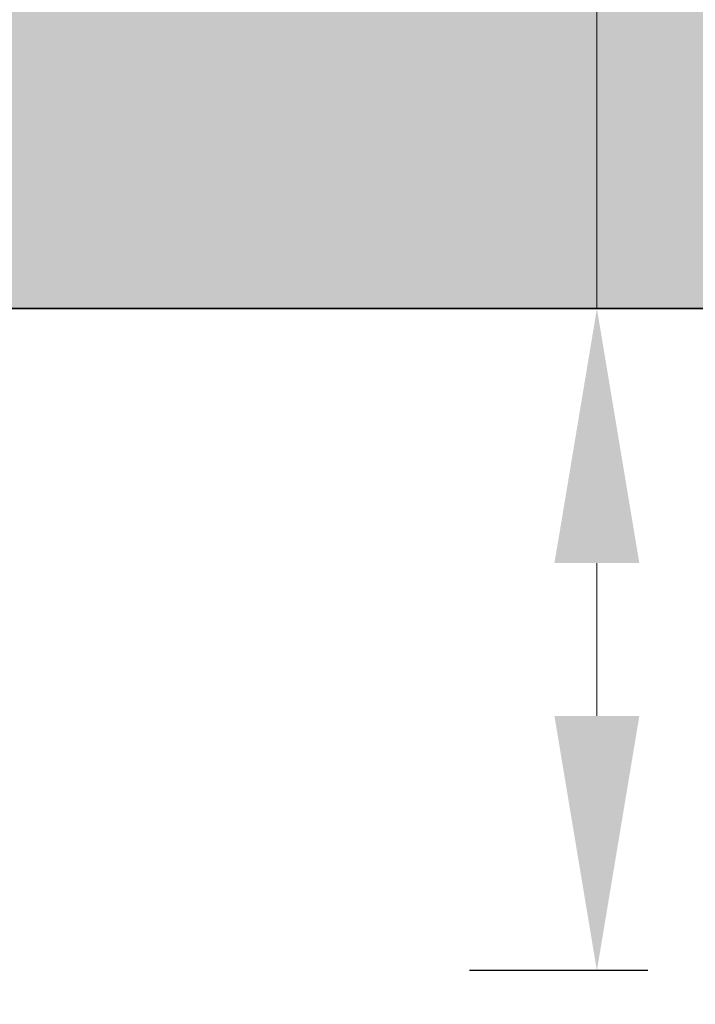
# Model space of a CAD drawing. Units: inches. Extents: x 2696 to 3240, y 1564 to 2310.
# Tile 43 of 76: x 2770.475 to 2777.108, y 2084.368 to 2094.037. Entities that reach past the tile are written whole.
import ezdxf

# ---------------------------------------------------------------- set-up
doc = ezdxf.new("R2010")
doc.units = ezdxf.units.IN
for name, color, linetype, lineweight in [('A-ANNO-DIMS', 3, 'Continuous', 18), ('A-WALL', 7, 'Continuous', 35), ('A-WALL-PATT', 9, 'Continuous', 13)]:
    doc.layers.add(name, color=color, linetype=linetype, lineweight=lineweight)
doc.styles.add('TIMES NEW', font='times.ttf')
doc.dimstyles.new('Siddhuu', dxfattribs={"dimtxt": 6, "dimasz": 2.5, "dimexe": 1.25, "dimexo": 0.625, "dimtad": 1, "dimdec": 1, "dimlunit": 4, "dimtxsty": 'TIMES NEW', "dimcen": 2.5, "dimclrd": 256, "dimclre": 1, "dimclrt": 7, "dimadec": 0, "dimazin": 0, "dimtfac": 1, "dimtdec": 1, "dimtmove": 0, "dimatfit": 3, "dimfxl": 1, "dimtolj": 1, "dimlwd": -1, "dimarcsym": 0})

# ---------------------------------------------------------------- blocks, each defined once
blk = doc.blocks.new('*D41')
at = {"layer": 'A-ANNO-DIMS', "transparency": 16777216}
for p, q in [((2776.1416, 2091.2011), (2776.1416, 2145.7283)), ((2776.1416, 2087.1996), (2776.1416, 2088.7011))]:
    blk.add_line(p, q, dxfattribs=at)
at = {"layer": 'A-ANNO-DIMS', "color": 1, "lineweight": -2, "transparency": 16777216}
for p, q in [((2776.6412, 2091.2011), (2774.8916, 2091.2011)), ((2776.6412, 2084.6996), (2774.8916, 2084.6996))]:
    blk.add_line(p, q, dxfattribs=at)
at = {"layer": 'A-ANNO-DIMS', "transparency": 16777216}
for points in [[(2775.7249, 2088.7011), (2776.5582, 2088.7011), (2776.1416, 2091.2011)], [(2775.7249, 2087.1996), (2776.5582, 2087.1996), (2776.1416, 2084.6996)]]:
    blk.add_solid(points, dxfattribs=at)
at = {"layer": 'Defpoints', "color": 0, "transparency": 16777216}
for p in [(2776.1416, 2091.2011), (2777.2662, 2091.2011), (2777.2662, 2084.6996)]:
    blk.add_point(p, dxfattribs=at)
at = {"layer": 'A-ANNO-DIMS', "color": 7, "transparency": 16777216, "insert": (2772.3803, 2119.7147), "char_height": 6, "attachment_point": 5, "rotation": 90, "style": 'TIMES NEW'}
blk.add_mtext('\\A1;0\'-6 1/2" TYP.', dxfattribs=at)
blk = doc.blocks.new('*D62')
at = {"layer": 'A-ANNO-DIMS', "color": 1, "lineweight": -2, "transparency": 16777216}
for p, q in [((2965.0838, 2140.7011), (2709.3614, 2140.7011)), ((2965.0838, 2063.5906), (2709.3614, 2063.5906))]:
    blk.add_line(p, q, dxfattribs=at)
at = {"layer": 'A-ANNO-DIMS', "transparency": 16777216}
blk.add_line((2710.6114, 2066.0906), (2710.6114, 2138.2011), dxfattribs=at)
for points in [[(2710.1947, 2138.2011), (2711.0281, 2138.2011), (2710.6114, 2140.7011)], [(2710.1947, 2066.0906), (2711.0281, 2066.0906), (2710.6114, 2063.5906)]]:
    blk.add_solid(points, dxfattribs=at)
at = {"layer": 'Defpoints', "color": 0, "transparency": 16777216}
for p in [(2710.6114, 2140.7011), (2965.7088, 2140.7011), (2965.7088, 2063.5906)]:
    blk.add_point(p, dxfattribs=at)
at = {"layer": 'A-ANNO-DIMS', "color": 7, "transparency": 16777216, "insert": (2706.9345, 2102.1459), "char_height": 6, "attachment_point": 5, "rotation": 90, "style": 'TIMES NEW'}
blk.add_mtext('\\A1;6\'-5"', dxfattribs=at)
blk = doc.blocks.new('*D64')
at = {"layer": 'A-ANNO-DIMS', "color": 1, "lineweight": -2, "transparency": 16777216}
for p, q in [((3073.0838, 2206.7011), (2709.3614, 2206.7011)), ((3068.5838, 1989.2011), (2709.3614, 1989.2011))]:
    blk.add_line(p, q, dxfattribs=at)
at = {"layer": 'A-ANNO-DIMS', "transparency": 16777216}
blk.add_line((2710.6114, 1991.7011), (2710.6114, 2204.2011), dxfattribs=at)
for points in [[(2710.1947, 2204.2011), (2711.0281, 2204.2011), (2710.6114, 2206.7011)], [(2710.1947, 1991.7011), (2711.0281, 1991.7011), (2710.6114, 1989.2011)]]:
    blk.add_solid(points, dxfattribs=at)
at = {"layer": 'Defpoints', "color": 0, "transparency": 16777216}
for p in [(2710.6114, 2206.7011), (3073.7088, 2206.7011), (3069.2088, 1989.2011)]:
    blk.add_point(p, dxfattribs=at)
at = {"layer": 'A-ANNO-DIMS', "color": 7, "transparency": 16777216, "insert": (2706.8501, 2097.9511), "char_height": 6, "attachment_point": 5, "rotation": 90, "style": 'TIMES NEW'}
blk.add_mtext('\\A1;18\'-1 1/2"', dxfattribs=at)
blk = doc.blocks.new('*D66')
at = {"layer": 'A-ANNO-DIMS', "color": 1, "lineweight": -2, "transparency": 16777216}
for p, q in [((3077.5838, 2122.7011), (2709.3614, 2122.7011)), ((3077.5838, 2074.7011), (2709.3614, 2074.7011))]:
    blk.add_line(p, q, dxfattribs=at)
at = {"layer": 'A-ANNO-DIMS', "transparency": 16777216}
blk.add_line((2710.6114, 2077.2011), (2710.6114, 2120.2011), dxfattribs=at)
for points in [[(2710.1947, 2120.2011), (2711.0281, 2120.2011), (2710.6114, 2122.7011)], [(2710.1947, 2077.2011), (2711.0281, 2077.2011), (2710.6114, 2074.7011)]]:
    blk.add_solid(points, dxfattribs=at)
at = {"layer": 'Defpoints', "color": 0, "transparency": 16777216}
for p in [(2710.6114, 2122.7011), (3078.2088, 2122.7011), (3078.2088, 2074.7011)]:
    blk.add_point(p, dxfattribs=at)
at = {"layer": 'A-ANNO-DIMS', "color": 7, "transparency": 16777216, "insert": (2706.9345, 2098.7011), "char_height": 6, "attachment_point": 5, "rotation": 90, "style": 'TIMES NEW'}
blk.add_mtext('\\A1;4\'-0"', dxfattribs=at)
blk = doc.blocks.new('*D68')
at = {"layer": 'A-ANNO-DIMS', "color": 1, "lineweight": -2, "transparency": 16777216}
for p, q in [((2745.6114, 2261.5761), (2745.6114, 1568.9511)), ((2782.8338, 2261.5761), (2782.8338, 1568.9511))]:
    blk.add_line(p, q, dxfattribs=at)
at = {"layer": 'A-ANNO-DIMS', "transparency": 16777216}
blk.add_line((2748.1114, 1570.2011), (2780.3338, 1570.2011), dxfattribs=at)
for points in [[(2748.1114, 1570.6178), (2748.1114, 1569.7844), (2745.6114, 1570.2011)], [(2780.3338, 1570.6178), (2780.3338, 1569.7844), (2782.8338, 1570.2011)]]:
    blk.add_solid(points, dxfattribs=at)
at = {"layer": 'Defpoints', "color": 0, "transparency": 16777216}
for p in [(2745.6114, 2262.2011), (2782.8338, 2262.2011), (2782.8338, 1570.2011)]:
    blk.add_point(p, dxfattribs=at)
at = {"layer": 'A-ANNO-DIMS', "color": 7, "transparency": 16777216, "insert": (2764.2226, 1573.878), "char_height": 6, "attachment_point": 5, "style": 'TIMES NEW'}
blk.add_mtext('\\A1;3\'-1"', dxfattribs=at)

msp = doc.modelspace()

# ---------------------------------------------------------------- hatches: boundary and pattern name
at = {"layer": 'A-WALL-PATT', "transparency": 33554556}
h = msp.add_hatch(color=256, dxfattribs=at)
h.dxf.hatch_style = 1
h.paths.add_polyline_path([(2879.1114, 2253.2011), (2905.9101, 2253.2011), (2905.9101, 2262.2011), (2841.889, 2262.2011), (2841.889, 2253.2011), (2870.1114, 2253.2011), (2870.1114, 2176.6011), (2965.7088, 2176.6011), (2965.7088, 2206.7011), (2973.5828, 2206.7011), (2973.5828, 2215.7011), (2965.7088, 2215.7011), (2965.7088, 2262.2011), (2929.9101, 2262.2011), (2929.9101, 2253.2011), (2956.7088, 2253.2011), (2956.7088, 2185.6011), (2879.1114, 2185.6011)])
h.paths.add_polyline_path([(2782.8338, 2262.2011), (2745.6114, 2262.2011), (2745.6114, 2228.7287), (2754.6114, 2228.7287), (2754.6114, 2253.2011), (2782.8338, 2253.2011)])
h.paths.add_polyline_path([(2754.6114, 2136.2011), (2965.7088, 2136.2011), (2965.7088, 2145.2011), (2879.1114, 2145.2011), (2879.1114, 2147.0735), (2877.3397, 2147.0735), (2870.1114, 2147.0735), (2870.1114, 2145.2011), (2754.6114, 2145.2011), (2754.6114, 2169.6735), (2745.6114, 2169.6735), (2745.6114, 2000.2011), (2754.6114, 2000.2011), (2754.6114, 2019.2011), (2849.0828, 2019.2011), (2849.0828, 2023.7011), (2841.2088, 2023.7011), (2841.2088, 2051.8271), (2836.7088, 2051.8271), (2836.7088, 2023.7011), (2754.6114, 2023.7011), (2754.6114, 2091.2011), (2836.7088, 2091.2011), (2836.7088, 2087.8271), (2841.2088, 2087.8271), (2841.2088, 2095.7011), (2754.6114, 2095.7011)])
h.paths.add_polyline_path([(2965.7088, 2136.2011), (2956.7088, 2136.2011), (2956.7088, 2023.7011), (2885.0828, 2023.7011), (2885.0828, 2019.2011), (2956.7088, 2019.2011), (2956.7088, 1950.5751), (2965.7088, 1950.5751), (2965.7088, 1980.2011), (2973.5828, 1980.2011), (2973.5828, 1989.2011), (2965.7088, 1989.2011)])
h.paths.add_polyline_path([(2754.6114, 1906.7011), (2880.2088, 1906.7011), (2884.7088, 1906.7011), (2956.7088, 1906.7011), (2956.7088, 1792.7011), (2944.7088, 1792.7011), (2944.7088, 1783.7011), (2956.7088, 1783.7011), (2956.7088, 1740.2011), (2884.7088, 1740.2011), (2884.7088, 1783.7011), (2896.7088, 1783.7011), (2896.7088, 1792.7011), (2884.7088, 1792.7011), (2884.7088, 1846.7011), (2880.2088, 1846.7011), (2880.2088, 1740.2011), (2754.6114, 1740.2011), (2754.6114, 1777.2011), (2745.6114, 1777.2011), (2745.6114, 1692.7011), (2754.6114, 1692.7011), (2754.6114, 1731.2011), (2956.7088, 1731.2011), (2956.7088, 1723.3271), (2965.7088, 1723.3271), (2965.7088, 1884.2011), (2973.5828, 1884.2011), (2973.5828, 1893.2011), (2965.7088, 1893.2011), (2965.7088, 1914.5751), (2956.7088, 1914.5751), (2956.7088, 1911.2011), (2754.6114, 1911.2011), (2754.6114, 1930.2011), (2745.6114, 1930.2011), (2745.6114, 1817.2011), (2754.6114, 1817.2011), (2754.6114, 1854.2011), (2826.6114, 1854.2011), (2826.6114, 1868.8271), (2822.1114, 1868.8271), (2822.1114, 1858.7011), (2754.6114, 1858.7011)])
h.paths.add_polyline_path([(2965.7088, 1656.2011), (3008.2374, 1656.2011), (3008.2374, 1665.2011), (2965.7088, 1665.2011), (2965.7088, 1693.3271), (2956.7088, 1693.3271), (2956.7088, 1686.2011), (2934.5828, 1686.2011), (2934.5828, 1681.7011), (2956.7088, 1681.7011), (2956.7088, 1614.2011), (2896.7088, 1614.2011), (2896.7088, 1681.7011), (2904.5828, 1681.7011), (2904.5828, 1686.2011), (2892.2088, 1686.2011), (2892.2088, 1614.2011), (2858.4101, 1614.2011), (2858.4101, 1605.2011), (2965.7088, 1605.2011)])
h.paths.add_polyline_path([(2788.4101, 1614.2011), (2754.6114, 1614.2011), (2754.6114, 1652.7011), (2745.6114, 1652.7011), (2745.6114, 1605.2011), (2788.4101, 1605.2011)])
h.paths.add_polyline_path([(3199.6114, 1633.0476), (3190.6114, 1633.0476), (3190.6114, 1614.2011), (3082.6114, 1614.2011), (3082.6114, 1665.2011), (3070.2374, 1665.2011), (3070.2374, 1656.2011), (3078.1114, 1656.2011), (3078.1114, 1605.2011), (3199.6114, 1605.2011)])
h.paths.add_polyline_path([(3199.6114, 1702.0476), (3190.6114, 1702.0476), (3190.6114, 1699.7011), (3106.6114, 1699.7011), (3106.6114, 1747.7011), (3190.6114, 1747.7011), (3190.6114, 1752.2011), (3082.6114, 1752.2011), (3082.6114, 1760.0751), (3078.1114, 1760.0751), (3078.1114, 1747.7011), (3102.1114, 1747.7011), (3102.1114, 1699.7011), (3078.1114, 1699.7011), (3078.1114, 1695.2011), (3190.6114, 1695.2011), (3190.6114, 1676.3546), (3199.6114, 1676.3546)])
h.paths.add_polyline_path([(3199.6114, 1783.2011), (3190.6114, 1783.2011), (3190.6114, 1745.3546), (3199.6114, 1745.3546)])
h.paths.add_polyline_path([(3082.6114, 1884.2011), (3190.6114, 1884.2011), (3190.6114, 1853.2011), (3199.6114, 1853.2011), (3199.6114, 1901.7011), (3190.6114, 1901.7011), (3190.6114, 1893.2011), (3005.5828, 1893.2011), (3005.5828, 1891.2811), (3005.5828, 1884.2011), (3078.1114, 1884.2011), (3078.1114, 1792.0751), (3082.6114, 1792.0751)])
h.paths.add_polyline_path([(3199.6114, 1994.7011), (3190.6114, 1994.7011), (3190.6114, 1989.2011), (3073.7088, 1989.2011), (3073.7088, 2034.2011), (3069.2088, 2034.2011), (3069.2088, 1989.2011), (3005.5828, 1989.2011), (3005.5828, 1980.2011), (3190.6114, 1980.2011), (3190.6114, 1971.7011), (3199.6114, 1971.7011)])
h.paths.add_polyline_path([(3199.6114, 2155.2011), (3190.6114, 2155.2011), (3190.6114, 2064.7011), (3199.6114, 2064.7011)])
h.paths.add_polyline_path([(3190.6114, 2074.7011), (3106.6114, 2074.7011), (3106.6114, 2122.7011), (3190.6114, 2122.7011), (3190.6114, 2127.2011), (3082.7088, 2127.2011), (3082.7088, 2135.0751), (3073.7088, 2135.0751), (3073.7088, 2122.7011), (3102.1114, 2122.7011), (3102.1114, 2074.7011), (3069.2088, 2074.7011), (3069.2088, 2070.2011), (3190.6114, 2070.2011)])
h.paths.add_polyline_path([(3082.7088, 2253.2011), (3190.6114, 2253.2011), (3190.6114, 2225.2011), (3199.6114, 2225.2011), (3199.6114, 2262.2011), (3073.7088, 2262.2011), (3073.7088, 2215.7011), (3035.5828, 2215.7011), (3035.5828, 2206.7011), (3073.7088, 2206.7011), (3073.7088, 2171.0751), (3082.7088, 2171.0751)])

# ---------------------------------------------------------------- linework, layer by layer
at = {"layer": 'A-WALL'}
msp.add_line((2754.6114, 2091.2011), (2836.7088, 2091.2011), dxfattribs=at)

# ---------------------------------------------------------------- dimensions: what is measured, and where the dimension line sits
at = {"layer": 'A-ANNO-DIMS'}
dim = msp.add_linear_dim(base=(2782.8338, 1570.2011), p1=(2745.6114, 2262.2011), p2=(2782.8338, 2262.2011), dimstyle='Siddhuu', override={"dimdec": 1, "dimlfac": 1, "dimrnd": 0, "dimzin": 1, "dimdsep": 46, "dimlunit": 4, "dimfrac": 2}, dxfattribs=at)
dim.commit()
dim.dimension.update_dxf_attribs({"geometry": '*D68', "text_midpoint": (2764.2226, 1573.878)})
for base, p1, p2, picture, middle in [((2710.6114, 2206.7011), (3069.2088, 1989.2011), (3073.7088, 2206.7011), '*D64', (2706.8501, 2097.9511)), ((2710.6114, 2140.7011), (2965.7088, 2063.5906), (2965.7088, 2140.7011), '*D62', (2706.9345, 2102.1459)), ((2710.6114, 2122.7011), (3078.2088, 2074.7011), (3078.2088, 2122.7011), '*D66', (2706.9345, 2098.7011))]:
    dim = msp.add_linear_dim(base=base, p1=p1, p2=p2, angle=90, dimstyle='Siddhuu', override={"dimdec": 1, "dimlfac": 1, "dimrnd": 0, "dimzin": 1, "dimdsep": 46, "dimlunit": 4, "dimfrac": 2}, dxfattribs=at)
    dim.commit()
    dim.dimension.update_dxf_attribs({"geometry": picture, "text_midpoint": middle})
dim = msp.add_linear_dim(base=(2776.1416, 2091.2011), p1=(2777.2662, 2084.6996), p2=(2777.2662, 2091.2011), angle=90, text='<> TYP.', dimstyle='Siddhuu', override={"dimdec": 1, "dimlfac": 1, "dimrnd": 0, "dimzin": 1, "dimdsep": 46, "dimlunit": 4, "dimfrac": 2}, dxfattribs=at)
dim.commit()
dim.dimension.update_dxf_attribs({"geometry": '*D41', "text_midpoint": (2772.3803, 2119.7147)})

doc.saveas('drawing.dxf')
